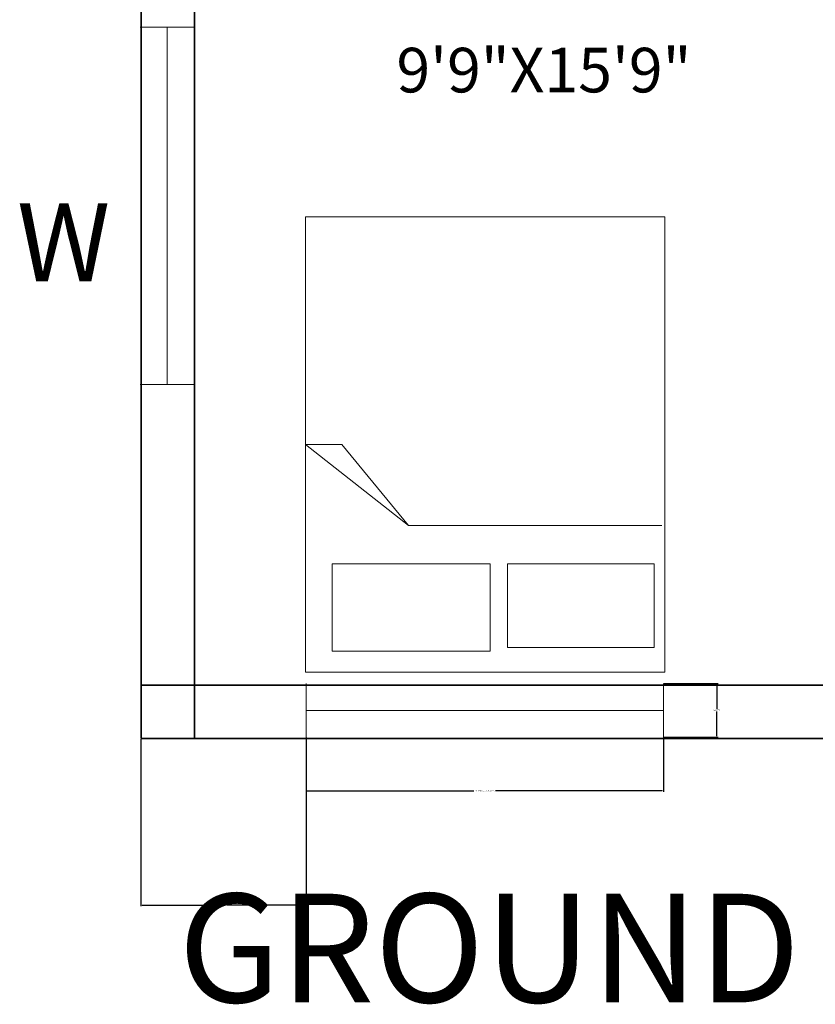
# Model space of a CAD drawing. Units: inches. Extents: x -26 to 788, y -42 to 505.
# Tile 1 of 9: x -17 to 116, y -42 to 123. Entities that reach past the tile are written whole.
import ezdxf

# ---------------------------------------------------------------- set-up
doc = ezdxf.new("R2010")
doc.units = ezdxf.units.IN
doc.header["$MEASUREMENT"] = 0
for name, color, linetype, lineweight in [('A-ANNO-DIMS', 2, 'Continuous', 18), ('A-ANNO-IDEN', 3, 'Continuous', 18), ('A-ANNO-TEXT', 7, 'Continuous', 25), ('A-AREA-IDEN', 7, 'Continuous', 18), ('A-FURN', 8, 'Continuous', 18), ('A-GLAZ', 4, 'Continuous', 18), ('A-WALL', 7, 'Continuous', 35)]:
    doc.layers.add(name, color=color, linetype=linetype, lineweight=lineweight)
doc.styles.get("Standard").update_dxf_attribs({"font": 'arial.ttf'})
doc.dimstyles.get("Standard").update_dxf_attribs({"dimtxt": 0.18, "dimasz": 0.18, "dimexe": 0.18, "dimexo": 0.0625, "dimgap": 0.09, "dimtad": 0, "dimtih": 1, "dimtoh": 1, "dimdec": 4, "dimzin": 0, "dimdsep": 46, "dimtxsty": 'Standard', "dimcen": 0.09, "dimadec": 0, "dimazin": 0, "dimtfac": 1, "dimtdec": 4, "dimtofl": 0, "dimtmove": 0, "dimatfit": 3, "dimfxl": 1, "dimtolj": 1, "dimtzin": 0, "dimarcsym": 0})

# ---------------------------------------------------------------- blocks, each defined once
blk = doc.blocks.new('WIN-SLIDER-60')
for p, q in [((0, 9), (0, 0)), ((60, 9), (60, 0)), ((0, 4.5), (60, 4.5)), ((60, 4.5), (50.65, 4.5))]:
    blk.add_line(p, q)
blk = doc.blocks.new('WIN-FIXED-60')
for p, q in [((0, 9), (0, 0)), ((60, 9), (60, 0)), ((0, 4.5), (60, 4.5))]:
    blk.add_line(p, q)
blk = doc.blocks.new('BED-DOUBLE')
for p, q in [((17.3, 24.61), (0, 38.23)), ((0, 38.23), (6.1, 38.23)), ((6.1, 38.23), (17.3, 24.61)), ((59.83, 24.61), (17.3, 24.61))]:
    blk.add_line(p, q)
for points in [[(0, 0), (60.34, 0), (60.34, 76.46), (0, 76.46)], [(4.51, 18.22), (31.05, 18.22), (31.05, 3.53), (4.51, 3.53)], [(33.93, 18.22), (58.56, 18.22), (58.56, 4.17), (33.93, 4.17)]]:
    blk.add_lwpolyline(points, close=True)
blk = doc.blocks.new('*D33')
at = {"layer": 'A-ANNO-DIMS', "color": 0, "lineweight": -2, "transparency": 16777216}
for p, q in [((30.67, 2.31), (30.67, -6.81)), ((90.67, 2.31), (90.67, -6.81)), ((30.85, -6.63), (58.84, -6.63)), ((90.49, -6.63), (62.5, -6.63))]:
    blk.add_line(p, q, dxfattribs=at)
at = {"layer": 'A-ANNO-DIMS', "color": 0, "transparency": 16777216}
for points in [[(30.85, -6.6), (30.85, -6.66), (30.67, -6.63)], [(90.49, -6.6), (90.49, -6.66), (90.67, -6.63)]]:
    blk.add_solid(points, dxfattribs=at)
at = {"layer": 'Defpoints', "color": 0, "transparency": 16777216}
for p in [(30.67, 2.37), (90.67, 2.37), (90.67, -6.63)]:
    blk.add_point(p, dxfattribs=at)
at = {"layer": 'A-ANNO-DIMS', "color": 0, "transparency": 16777216, "insert": (60.67, -6.63), "char_height": 0.18, "attachment_point": 5}
blk.add_mtext('\\A1;FIXED WINDOW 60.0000 TYP.', dxfattribs=at)
blk = doc.blocks.new('*D34')
at = {"layer": 'A-ANNO-DIMS', "color": 0, "lineweight": -2, "transparency": 16777216}
for p, q in [((90.73, 11.37), (99.85, 11.37)), ((99.67, 11.19), (99.67, 7.05)), ((99.67, 2.55), (99.67, 6.69)), ((90.73, 2.37), (99.85, 2.37))]:
    blk.add_line(p, q, dxfattribs=at)
at = {"layer": 'A-ANNO-DIMS', "color": 0, "transparency": 16777216}
for points in [[(99.64, 11.19), (99.7, 11.19), (99.67, 11.37)], [(99.64, 2.55), (99.7, 2.55), (99.67, 2.37)]]:
    blk.add_solid(points, dxfattribs=at)
at = {"layer": 'Defpoints', "color": 0, "transparency": 16777216}
for p in [(90.67, 11.37), (99.67, 11.37), (90.67, 2.37)]:
    blk.add_point(p, dxfattribs=at)
at = {"layer": 'A-ANNO-DIMS', "color": 0, "transparency": 16777216, "insert": (99.67, 6.87), "char_height": 0.18, "attachment_point": 5}
blk.add_mtext('\\A1;9.0000 TYP.', dxfattribs=at)
blk = doc.blocks.new('*D56')
at = {"layer": 'A-ANNO-DIMS', "color": 0, "lineweight": -2, "transparency": 16777216}
for p, q in [((2.95, 2.06), (2.95, -26.01)), ((30.67, 2.31), (30.67, -26.01)), ((3.13, -25.83), (16.28, -25.83)), ((30.49, -25.83), (17.35, -25.83))]:
    blk.add_line(p, q, dxfattribs=at)
at = {"layer": 'A-ANNO-DIMS', "color": 0, "transparency": 16777216}
for points in [[(3.13, -25.8), (3.13, -25.86), (2.95, -25.83)], [(30.49, -25.8), (30.49, -25.86), (30.67, -25.83)]]:
    blk.add_solid(points, dxfattribs=at)
at = {"layer": 'Defpoints', "color": 0, "transparency": 16777216}
for p in [(2.95, 2.12), (30.67, 2.37), (30.67, -25.83)]:
    blk.add_point(p, dxfattribs=at)
at = {"layer": 'A-ANNO-DIMS', "color": 0, "transparency": 16777216, "insert": (16.81, -25.83), "char_height": 0.18, "attachment_point": 5}
blk.add_mtext('\\A1;27.7127', dxfattribs=at)

msp = doc.modelspace()

# ---------------------------------------------------------------- linework, layer by layer
at = {"layer": 'A-WALL'}
for p, q in [((2.95497, 2.11777), (2.95497, 431.11777)), ((11.95497, 2.11777), (11.95497, 260.11777)), ((2.95497, 11.11777), (307.45497, 11.11777)), ((2.95497, 2.11777), (307.45497, 2.11777))]:
    msp.add_line(p, q, dxfattribs=at)

# ---------------------------------------------------------------- block references
at = {"layer": 'A-FURN'}
msp.add_blockref('BED-DOUBLE', (30.552, 13.263), dxfattribs=at)
at = {"layer": 'A-GLAZ', "rotation": 270}
msp.add_blockref('WIN-SLIDER-60', (2.82682, 121.53152), dxfattribs=at)
at = {"layer": 'A-GLAZ'}
msp.add_blockref('WIN-FIXED-60', (30.668, 2.372), dxfattribs=at)

# ---------------------------------------------------------------- texts
at = {"layer": 'A-ANNO-IDEN'}
msp.add_text('W', height=13.09317, dxfattribs=at).set_placement((-17.88113, 78.89311))
at = {"layer": 'A-ANNO-TEXT'}
msp.add_text('GROUND FLOOR PLAN', height=18.2344212, dxfattribs=at).set_placement((9.22807, -42.14293))
at = {"layer": 'A-AREA-IDEN'}
msp.add_text('9\'9"X15\'9"', height=7.483862, dxfattribs=at).set_placement((45.84217, 110.58161))

# ---------------------------------------------------------------- dimensions: what is measured, and where the dimension line sits
at = {"layer": 'A-ANNO-DIMS'}
dim = msp.add_linear_dim(base=(99.6677, 11.37181), p1=(90.6677, 2.37181), p2=(90.6677, 11.37181), angle=90, text='<> TYP.', dimstyle='Standard', override={"dimdec": 4, "dimlfac": 1, "dimrnd": 0, "dimzin": 0, "dimdsep": 46, "dimlunit": 2}, dxfattribs=at)
dim.commit()
dim.dimension.update_dxf_attribs({"geometry": '*D34', "text_midpoint": (99.6677, 6.87181)})
dim = msp.add_linear_dim(base=(30.6677, -25.83223), p1=(2.95497, 2.11777), p2=(30.6677, 2.37181), dimstyle='Standard', override={"dimdec": 4, "dimlfac": 1, "dimrnd": 0, "dimzin": 0, "dimdsep": 46, "dimlunit": 2}, dxfattribs=at)
dim.commit()
dim.dimension.update_dxf_attribs({"geometry": '*D56', "text_midpoint": (16.81133, -25.83223)})
dim = msp.add_linear_dim(base=(90.6677, -6.62819), p1=(30.6677, 2.37181), p2=(90.6677, 2.37181), text='FIXED WINDOW <> TYP.', dimstyle='Standard', override={"dimdec": 4, "dimlfac": 1, "dimrnd": 0, "dimzin": 0, "dimdsep": 46, "dimlunit": 2}, dxfattribs=at)
dim.commit()
dim.dimension.update_dxf_attribs({"geometry": '*D33', "text_midpoint": (60.6677, -6.62819)})

doc.saveas('drawing.dxf')
